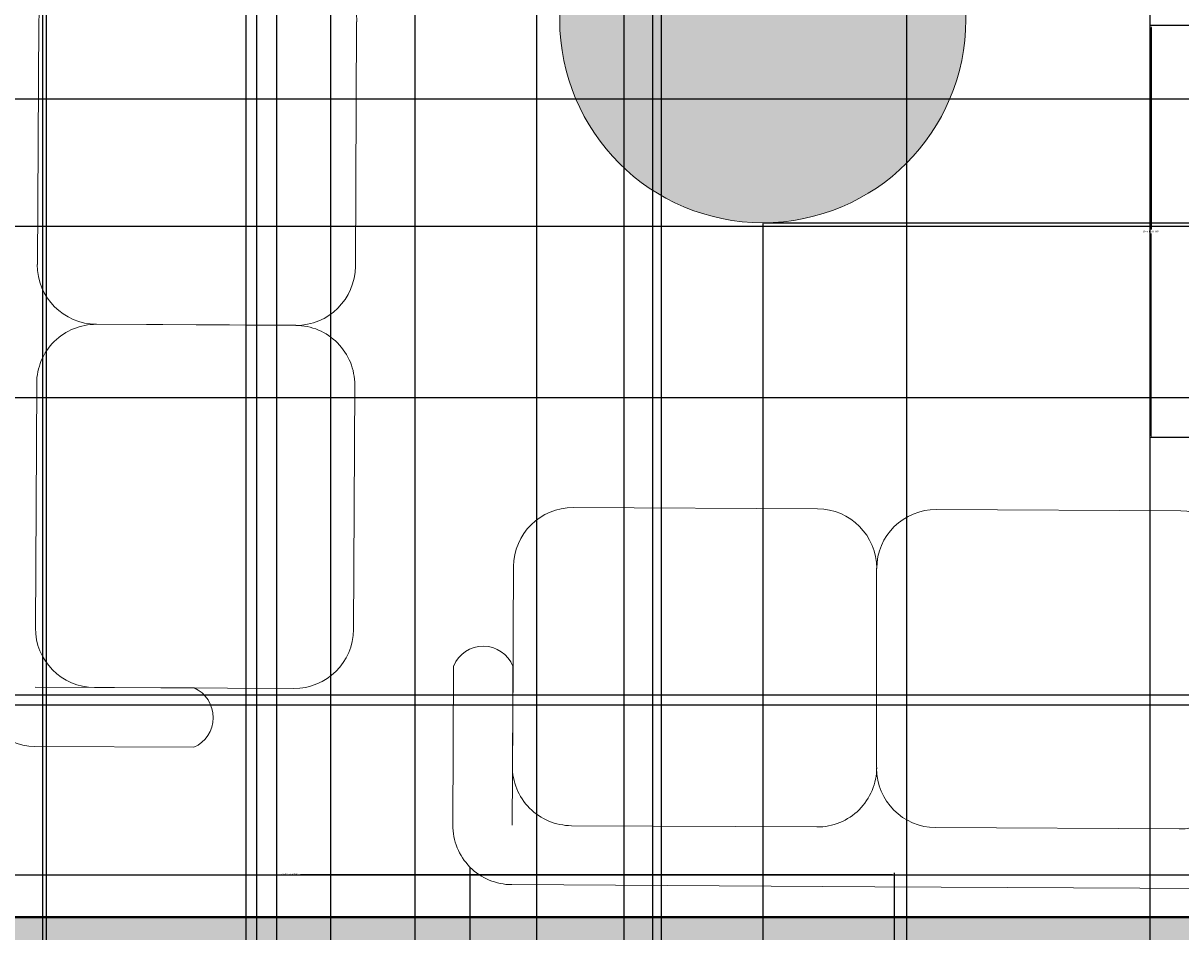
# Model space of a CAD drawing. Units: inches. Extents: x 818 to 1898, y 976 to 2364.
# Tile 32 of 96: x 1282 to 1391, y 1695 to 1780. Entities that reach past the tile are written whole.
import ezdxf

# ---------------------------------------------------------------- set-up
doc = ezdxf.new("R2010")
doc.units = ezdxf.units.IN
doc.header["$LTSCALE"] = 5
doc.header["$MEASUREMENT"] = 0
for name, color, linetype, lineweight in [('A-ANNO-DIMS', 2, 'Continuous', 18), ('A-FLOR-CASE-PATT', 33, 'Continuous', 9), ('A-FURN', 8, 'Continuous', 18), ('A-WALL', 7, 'Continuous', 40)]:
    doc.layers.add(name, color=color, linetype=linetype, lineweight=lineweight)
doc.layers.add('A-WALL-PATT', color=251, linetype='Continuous', lineweight=13, true_color=0x636466)
doc.styles.get("Standard").update_dxf_attribs({"font": 'arial.ttf'})
doc.dimstyles.get("Standard").update_dxf_attribs({"dimtxt": 0.18, "dimasz": 0.18, "dimexe": 0.18, "dimexo": 0.0625, "dimgap": 0.09, "dimtad": 0, "dimtih": 1, "dimtoh": 1, "dimdec": 4, "dimzin": 0, "dimdsep": 46, "dimtxsty": 'Standard', "dimcen": 0.09, "dimadec": 0, "dimazin": 0, "dimtfac": 1, "dimtdec": 4, "dimtofl": 0, "dimtmove": 0, "dimatfit": 3, "dimfxl": 1, "dimtolj": 1, "dimtzin": 0, "dimarcsym": 0})

# ---------------------------------------------------------------- blocks, each defined once
blk = doc.blocks.new('SOFA-3-SEAT')
for p, q in [((39.87, 35.86), (5.7, 36.05)), ((74.05, 35.68), (39.88, 35.86)), ((108.23, 35.49), (74.06, 35.68)), ((0, 15.52), (0.08, 30.49)), ((5.59, 15.49), (5.67, 30.46)), ((34.25, 30.31), (11.25, 30.43)), ((68.34, 30.12), (45.43, 30.24)), ((102.62, 29.94), (79.51, 30.06)), ((108.12, 14.94), (108.2, 29.9)), ((113.71, 14.91), (113.79, 29.87)), ((5.64, 24.87), (5.54, 6.11)), ((39.71, 5.93), (39.81, 24.69)), ((39.82, 24.69), (39.72, 5.93)), ((73.9, 5.71), (73.9, 24.47)), ((108.07, 5.56), (108.17, 24.32)), ((11.09, 0.49), (34.09, 0.37)), ((45.27, 0.31), (68.27, 0.19)), ((79.45, 0.12), (102.45, 0))]:
    blk.add_line(p, q)
for centre, radius, start, end in [((5.67, 30.46), 5.59, 89.6898, 179.6898), ((108.2, 29.9), 5.59, 359.6898, 89.6898), ((11.22, 24.84), 5.59, 89.6898, 179.6898), ((34.22, 24.72), 5.59, 359.6898, 89.6898), ((45.4, 24.66), 5.59, 89.6898, 179.6898), ((68.31, 24.53), 5.59, 0, 89.6898), ((79.48, 24.47), 5.59, 89.6898, 180), ((102.59, 24.35), 5.59, 359.6898, 89.6898), ((2.8, 16.75), 3.06, 203.7099, 335.6698), ((110.92, 16.05), 3.01, 201.7034, 337.6762), ((11.12, 6.08), 5.59, 179.6898, 269.6898), ((34.12, 5.96), 5.59, 269.6898, 359.6898), ((45.3, 5.9), 5.59, 179.6898, 269.6898), ((68.3, 5.77), 5.59, 269.6898, 359.6898), ((79.48, 5.71), 5.59, 179.6898, 269.6898), ((102.48, 5.59), 5.59, 269.6898, 359.6898)]:
    blk.add_arc(centre, radius, start, end)
blk = doc.blocks.new('*D42')
at = {"layer": 'A-ANNO-DIMS', "color": 0, "lineweight": -2, "ltscale": 5, "transparency": 16777216}
for p, q in [((1250.19, 1683.07), (1250.19, 1700.26)), ((1250.37, 1700.08), (1306.12, 1700.08)), ((1363.82, 1700.08), (1308.07, 1700.08)), ((1364, 1683.07), (1364, 1700.26))]:
    blk.add_line(p, q, dxfattribs=at)
at = {"layer": 'A-ANNO-DIMS', "color": 0, "ltscale": 5, "transparency": 16777216}
for points in [[(1250.37, 1700.11), (1250.37, 1700.05), (1250.19, 1700.08)], [(1363.82, 1700.11), (1363.82, 1700.05), (1364, 1700.08)]]:
    blk.add_solid(points, dxfattribs=at)
at = {"layer": 'Defpoints', "color": 0, "ltscale": 5, "transparency": 16777216}
for p in [(1364, 1700.08), (1250.19, 1683.01), (1364, 1683.01)]:
    blk.add_point(p, dxfattribs=at)
at = {"layer": 'A-ANNO-DIMS', "color": 0, "ltscale": 5, "transparency": 16777216, "insert": (1307.1, 1700.08), "char_height": 0.18, "attachment_point": 5}
blk.add_mtext('\\A1;SOFA 114 TYP.', dxfattribs=at)
blk = doc.blocks.new('*D50')
at = {"layer": 'A-ANNO-DIMS', "color": 0, "lineweight": -2, "ltscale": 5, "transparency": 16777216}
for p, q in [((1393.92, 1780.01), (1387.99, 1780.01)), ((1388.17, 1779.83), (1388.17, 1760.8)), ((1388.17, 1741.4), (1388.17, 1760.43)), ((1393.92, 1741.22), (1387.99, 1741.22))]:
    blk.add_line(p, q, dxfattribs=at)
at = {"layer": 'A-ANNO-DIMS', "color": 0, "ltscale": 5, "transparency": 16777216}
for points in [[(1388.14, 1779.83), (1388.2, 1779.83), (1388.17, 1780.01)], [(1388.14, 1741.4), (1388.2, 1741.4), (1388.17, 1741.22)]]:
    blk.add_solid(points, dxfattribs=at)
at = {"layer": 'Defpoints', "color": 0, "ltscale": 5, "transparency": 16777216}
for p in [(1388.17, 1780.01), (1393.99, 1780.01), (1393.99, 1741.22)]:
    blk.add_point(p, dxfattribs=at)
at = {"layer": 'A-ANNO-DIMS', "color": 0, "ltscale": 5, "transparency": 16777216, "insert": (1388.17, 1760.62), "char_height": 0.18, "attachment_point": 5}
blk.add_mtext('\\A1;CHAIR 39 TYP.', dxfattribs=at)
blk = doc.blocks.new('*D61')
at = {"layer": 'A-ANNO-DIMS', "color": 0, "lineweight": -2, "ltscale": 5, "transparency": 16777216}
for p, q in [((1071.73, 1203.03), (1071.73, 2363.87)), ((1071.91, 2363.69), (1250.94, 2363.69)), ((1430.55, 2363.69), (1251.51, 2363.69)), ((1430.73, 1203.03), (1430.73, 2363.87))]:
    blk.add_line(p, q, dxfattribs=at)
at = {"layer": 'A-ANNO-DIMS', "color": 0, "ltscale": 5, "transparency": 16777216}
for points in [[(1071.91, 2363.72), (1071.91, 2363.66), (1071.73, 2363.69)], [(1430.55, 2363.72), (1430.55, 2363.66), (1430.73, 2363.69)]]:
    blk.add_solid(points, dxfattribs=at)
at = {"layer": 'Defpoints', "color": 0, "ltscale": 5, "transparency": 16777216}
for p in [(1430.73, 2363.69), (1071.73, 1202.96), (1430.73, 1202.96)]:
    blk.add_point(p, dxfattribs=at)
at = {"layer": 'A-ANNO-DIMS', "color": 0, "ltscale": 5, "transparency": 16777216, "insert": (1251.23, 2363.69), "char_height": 0.18, "attachment_point": 5}
blk.add_mtext('\\A1;359', dxfattribs=at)
blk = doc.blocks.new('*D64')
at = {"layer": 'A-ANNO-DIMS', "color": 0, "lineweight": -2, "ltscale": 5, "transparency": 16777216}
for p, q in [((1197.73, 1501.14), (1197.73, 2363.87)), ((1197.91, 2363.69), (1313.93, 2363.69)), ((1430.55, 2363.69), (1314.52, 2363.69)), ((1430.73, 1501.14), (1430.73, 2363.87))]:
    blk.add_line(p, q, dxfattribs=at)
at = {"layer": 'A-ANNO-DIMS', "color": 0, "ltscale": 5, "transparency": 16777216}
for points in [[(1197.91, 2363.72), (1197.91, 2363.66), (1197.73, 2363.69)], [(1430.55, 2363.72), (1430.55, 2363.66), (1430.73, 2363.69)]]:
    blk.add_solid(points, dxfattribs=at)
at = {"layer": 'Defpoints', "color": 0, "ltscale": 5, "transparency": 16777216}
for p in [(1430.73, 2363.69), (1197.73, 1501.08), (1430.73, 1501.08)]:
    blk.add_point(p, dxfattribs=at)
at = {"layer": 'A-ANNO-DIMS', "color": 0, "ltscale": 5, "transparency": 16777216, "insert": (1314.23, 2363.69), "char_height": 0.18, "attachment_point": 5}
blk.add_mtext('\\A1;233', dxfattribs=at)
blk = doc.blocks.new('*D85')
at = {"layer": 'A-ANNO-DIMS', "color": 0, "lineweight": -2, "ltscale": 5, "transparency": 16777216}
for p, q in [((1258.79, 2053.08), (1897.92, 2053.08)), ((1897.74, 2052.9), (1897.74, 1876.76)), ((1897.74, 1700.26), (1897.74, 1876.4)), ((1258.79, 1700.08), (1897.92, 1700.08))]:
    blk.add_line(p, q, dxfattribs=at)
at = {"layer": 'A-ANNO-DIMS', "color": 0, "ltscale": 5, "transparency": 16777216}
for points in [[(1897.71, 2052.9), (1897.77, 2052.9), (1897.74, 2053.08)], [(1897.71, 1700.26), (1897.77, 1700.26), (1897.74, 1700.08)]]:
    blk.add_solid(points, dxfattribs=at)
at = {"layer": 'Defpoints', "color": 0, "ltscale": 5, "transparency": 16777216}
for p in [(1258.73, 2053.08), (1897.74, 2053.08), (1258.73, 1700.08)]:
    blk.add_point(p, dxfattribs=at)
at = {"layer": 'A-ANNO-DIMS', "color": 0, "ltscale": 5, "transparency": 16777216, "insert": (1897.74, 1876.58), "char_height": 0.18, "attachment_point": 5}
blk.add_mtext('\\A1;353', dxfattribs=at)
blk = doc.blocks.new('*D96')
at = {"layer": 'A-ANNO-DIMS', "color": 0, "lineweight": -2, "ltscale": 5, "transparency": 16777216}
for p, q in [((1229.65, 1071.12), (1229.65, 2363.87)), ((1229.83, 2363.69), (1256.52, 2363.69)), ((1283.99, 2363.69), (1257.3, 2363.69)), ((1284.17, 1071.12), (1284.17, 2363.87))]:
    blk.add_line(p, q, dxfattribs=at)
at = {"layer": 'A-ANNO-DIMS', "color": 0, "ltscale": 5, "transparency": 16777216}
for points in [[(1229.83, 2363.72), (1229.83, 2363.66), (1229.65, 2363.69)], [(1283.99, 2363.72), (1283.99, 2363.66), (1284.17, 2363.69)]]:
    blk.add_solid(points, dxfattribs=at)
at = {"layer": 'Defpoints', "color": 0, "ltscale": 5, "transparency": 16777216}
for p in [(1284.17, 2363.69), (1229.65, 1071.06), (1284.17, 1071.06)]:
    blk.add_point(p, dxfattribs=at)
at = {"layer": 'A-ANNO-DIMS', "color": 0, "ltscale": 5, "transparency": 16777216, "insert": (1256.91, 2363.69), "char_height": 0.18, "attachment_point": 5}
blk.add_mtext('\\A1;54.52', dxfattribs=at)
blk = doc.blocks.new('*D97')
at = {"layer": 'A-ANNO-DIMS', "color": 0, "lineweight": -2, "ltscale": 5, "transparency": 16777216}
for p, q in [((1284.17, 1071.12), (1284.17, 2363.87)), ((1284.35, 2363.69), (1310.96, 2363.69)), ((1338.36, 2363.69), (1311.75, 2363.69)), ((1338.54, 1071.12), (1338.54, 2363.87))]:
    blk.add_line(p, q, dxfattribs=at)
at = {"layer": 'A-ANNO-DIMS', "color": 0, "ltscale": 5, "transparency": 16777216}
for points in [[(1284.35, 2363.72), (1284.35, 2363.66), (1284.17, 2363.69)], [(1338.36, 2363.72), (1338.36, 2363.66), (1338.54, 2363.69)]]:
    blk.add_solid(points, dxfattribs=at)
at = {"layer": 'Defpoints', "color": 0, "ltscale": 5, "transparency": 16777216}
for p in [(1338.54, 2363.69), (1284.17, 1071.06), (1338.54, 1071.06)]:
    blk.add_point(p, dxfattribs=at)
at = {"layer": 'A-ANNO-DIMS', "color": 0, "ltscale": 5, "transparency": 16777216, "insert": (1311.36, 2363.69), "char_height": 0.18, "attachment_point": 5}
blk.add_mtext('\\A1;54.37', dxfattribs=at)
blk = doc.blocks.new('*D98')
at = {"layer": 'A-ANNO-DIMS', "color": 0, "lineweight": -2, "ltscale": 5, "transparency": 16777216}
for p, q in [((1338.54, 1071.12), (1338.54, 2363.87)), ((1338.72, 2363.69), (1364.81, 2363.69)), ((1391.7, 2363.69), (1365.6, 2363.69)), ((1391.88, 1071.12), (1391.88, 2363.87))]:
    blk.add_line(p, q, dxfattribs=at)
at = {"layer": 'A-ANNO-DIMS', "color": 0, "ltscale": 5, "transparency": 16777216}
for points in [[(1338.72, 2363.72), (1338.72, 2363.66), (1338.54, 2363.69)], [(1391.7, 2363.72), (1391.7, 2363.66), (1391.88, 2363.69)]]:
    blk.add_solid(points, dxfattribs=at)
at = {"layer": 'Defpoints', "color": 0, "ltscale": 5, "transparency": 16777216}
for p in [(1391.88, 2363.69), (1338.54, 1071.06), (1391.88, 1071.06)]:
    blk.add_point(p, dxfattribs=at)
at = {"layer": 'A-ANNO-DIMS', "color": 0, "ltscale": 5, "transparency": 16777216, "insert": (1365.21, 2363.69), "char_height": 0.18, "attachment_point": 5}
blk.add_mtext('\\A1;53.33', dxfattribs=at)
blk = doc.blocks.new('*D119')
at = {"layer": 'A-ANNO-DIMS', "color": 0, "lineweight": -2, "ltscale": 5, "transparency": 16777216}
for p, q in [((1766.29, 1716.99), (818.03, 1716.99)), ((818.21, 1716.81), (818.21, 1672.43)), ((818.21, 1627.69), (818.21, 1672.06)), ((1766.29, 1627.51), (818.03, 1627.51))]:
    blk.add_line(p, q, dxfattribs=at)
at = {"layer": 'A-ANNO-DIMS', "color": 0, "ltscale": 5, "transparency": 16777216}
for points in [[(818.18, 1716.81), (818.24, 1716.81), (818.21, 1716.99)], [(818.18, 1627.69), (818.24, 1627.69), (818.21, 1627.51)]]:
    blk.add_solid(points, dxfattribs=at)
at = {"layer": 'Defpoints', "color": 0, "ltscale": 5, "transparency": 16777216}
for p in [(818.21, 1716.99), (1766.35, 1716.99), (1766.35, 1627.51)]:
    blk.add_point(p, dxfattribs=at)
at = {"layer": 'A-ANNO-DIMS', "color": 0, "ltscale": 5, "transparency": 16777216, "insert": (818.21, 1672.25), "char_height": 0.18, "attachment_point": 5}
blk.add_mtext('\\A1;89.48', dxfattribs=at)
blk = doc.blocks.new('*D120')
at = {"layer": 'A-ANNO-DIMS', "color": 0, "lineweight": -2, "ltscale": 5, "transparency": 16777216}
for p, q in [((1766.29, 1797.72), (818.03, 1797.72)), ((818.21, 1797.54), (818.21, 1757.53)), ((818.21, 1717.17), (818.21, 1757.17)), ((1766.29, 1716.99), (818.03, 1716.99))]:
    blk.add_line(p, q, dxfattribs=at)
at = {"layer": 'A-ANNO-DIMS', "color": 0, "ltscale": 5, "transparency": 16777216}
for points in [[(818.18, 1797.54), (818.24, 1797.54), (818.21, 1797.72)], [(818.18, 1717.17), (818.24, 1717.17), (818.21, 1716.99)]]:
    blk.add_solid(points, dxfattribs=at)
at = {"layer": 'Defpoints', "color": 0, "ltscale": 5, "transparency": 16777216}
for p in [(818.21, 1797.72), (1766.35, 1797.72), (1766.35, 1716.99)]:
    blk.add_point(p, dxfattribs=at)
at = {"layer": 'A-ANNO-DIMS', "color": 0, "ltscale": 5, "transparency": 16777216, "insert": (818.21, 1757.35), "char_height": 0.18, "attachment_point": 5}
blk.add_mtext('\\A1;80.73', dxfattribs=at)
blk = doc.blocks.new('*D165')
at = {"layer": 'A-ANNO-DIMS', "color": 0, "lineweight": -2, "ltscale": 5, "transparency": 16777216}
for p, q in [((1283.82, 1510.14), (1283.82, 2363.87)), ((1284, 2363.69), (1324.09, 2363.69)), ((1364.97, 2363.69), (1324.88, 2363.69)), ((1365.15, 1510.14), (1365.15, 2363.87))]:
    blk.add_line(p, q, dxfattribs=at)
at = {"layer": 'A-ANNO-DIMS', "color": 0, "ltscale": 5, "transparency": 16777216}
for points in [[(1284, 2363.72), (1284, 2363.66), (1283.82, 2363.69)], [(1364.97, 2363.72), (1364.97, 2363.66), (1365.15, 2363.69)]]:
    blk.add_solid(points, dxfattribs=at)
at = {"layer": 'Defpoints', "color": 0, "ltscale": 5, "transparency": 16777216}
for p in [(1365.15, 2363.69), (1283.82, 1510.08), (1365.15, 1510.08)]:
    blk.add_point(p, dxfattribs=at)
at = {"layer": 'A-ANNO-DIMS', "color": 0, "ltscale": 5, "transparency": 16777216, "insert": (1324.48, 2363.69), "char_height": 0.18, "attachment_point": 5}
blk.add_mtext('\\A1;81.33', dxfattribs=at)
blk = doc.blocks.new('*D215')
at = {"layer": 'A-ANNO-DIMS', "color": 0, "lineweight": -2, "ltscale": 5, "transparency": 16777216}
for p, q in [((1590.66, 1876.08), (818.03, 1876.08)), ((818.21, 1875.9), (818.21, 1781.76)), ((818.21, 1687.26), (818.21, 1781.4)), ((1511.66, 1687.08), (818.03, 1687.08))]:
    blk.add_line(p, q, dxfattribs=at)
at = {"layer": 'A-ANNO-DIMS', "color": 0, "ltscale": 5, "transparency": 16777216}
for points in [[(818.18, 1875.9), (818.24, 1875.9), (818.21, 1876.08)], [(818.18, 1687.26), (818.24, 1687.26), (818.21, 1687.08)]]:
    blk.add_solid(points, dxfattribs=at)
at = {"layer": 'Defpoints', "color": 0, "ltscale": 5, "transparency": 16777216}
for p in [(818.21, 1876.08), (1590.73, 1876.08), (1511.73, 1687.08)]:
    blk.add_point(p, dxfattribs=at)
at = {"layer": 'A-ANNO-DIMS', "color": 0, "ltscale": 5, "transparency": 16777216, "insert": (818.21, 1781.58), "char_height": 0.18, "attachment_point": 5}
blk.add_mtext('\\A1;189', dxfattribs=at)
blk = doc.blocks.new('*D220')
at = {"layer": 'A-ANNO-DIMS', "color": 0, "lineweight": -2, "ltscale": 5, "transparency": 16777216}
for p, q in [((1520.66, 1773.08), (818.03, 1773.08)), ((818.21, 1772.9), (818.21, 1767.26)), ((818.21, 1761.26), (818.21, 1766.9)), ((1520.66, 1761.08), (818.03, 1761.08))]:
    blk.add_line(p, q, dxfattribs=at)
at = {"layer": 'A-ANNO-DIMS', "color": 0, "ltscale": 5, "transparency": 16777216}
for points in [[(818.18, 1772.9), (818.24, 1772.9), (818.21, 1773.08)], [(818.18, 1761.26), (818.24, 1761.26), (818.21, 1761.08)]]:
    blk.add_solid(points, dxfattribs=at)
at = {"layer": 'Defpoints', "color": 0, "ltscale": 5, "transparency": 16777216}
for p in [(818.21, 1773.08), (1520.73, 1773.08), (1520.73, 1761.08)]:
    blk.add_point(p, dxfattribs=at)
at = {"layer": 'A-ANNO-DIMS', "color": 0, "ltscale": 5, "transparency": 16777216, "insert": (818.21, 1767.08), "char_height": 0.18, "attachment_point": 5}
blk.add_mtext('\\A1;12', dxfattribs=at)
blk = doc.blocks.new('*D222')
at = {"layer": 'A-ANNO-DIMS', "color": 0, "lineweight": -2, "ltscale": 5, "transparency": 16777216}
for p, q in [((1511.66, 1744.97), (818.03, 1744.97)), ((818.21, 1744.79), (818.21, 1730.69)), ((818.21, 1716.23), (818.21, 1730.33)), ((1511.66, 1716.05), (818.03, 1716.05))]:
    blk.add_line(p, q, dxfattribs=at)
at = {"layer": 'A-ANNO-DIMS', "color": 0, "ltscale": 5, "transparency": 16777216}
for points in [[(818.18, 1744.79), (818.24, 1744.79), (818.21, 1744.97)], [(818.18, 1716.23), (818.24, 1716.23), (818.21, 1716.05)]]:
    blk.add_solid(points, dxfattribs=at)
at = {"layer": 'Defpoints', "color": 0, "ltscale": 5, "transparency": 16777216}
for p in [(818.21, 1744.97), (1511.73, 1744.97), (1511.73, 1716.05)]:
    blk.add_point(p, dxfattribs=at)
at = {"layer": 'A-ANNO-DIMS', "color": 0, "ltscale": 5, "transparency": 16777216, "insert": (818.21, 1730.51), "char_height": 0.18, "attachment_point": 5}
blk.add_mtext('\\A1;28.926', dxfattribs=at)
blk = doc.blocks.new('*D223')
at = {"layer": 'A-ANNO-DIMS', "color": 0, "lineweight": -2, "ltscale": 5, "transparency": 16777216}
for p, q in [((1511.66, 1716.05), (818.03, 1716.05)), ((818.21, 1715.87), (818.21, 1706.24)), ((818.21, 1696.26), (818.21, 1705.88)), ((1511.66, 1696.08), (818.03, 1696.08))]:
    blk.add_line(p, q, dxfattribs=at)
at = {"layer": 'A-ANNO-DIMS', "color": 0, "ltscale": 5, "transparency": 16777216}
for points in [[(818.18, 1715.87), (818.24, 1715.87), (818.21, 1716.05)], [(818.18, 1696.26), (818.24, 1696.26), (818.21, 1696.08)]]:
    blk.add_solid(points, dxfattribs=at)
at = {"layer": 'Defpoints', "color": 0, "ltscale": 5, "transparency": 16777216}
for p in [(818.21, 1716.05), (1511.73, 1716.05), (1511.73, 1696.08)]:
    blk.add_point(p, dxfattribs=at)
at = {"layer": 'A-ANNO-DIMS', "color": 0, "ltscale": 5, "transparency": 16777216, "insert": (818.21, 1706.06), "char_height": 0.18, "attachment_point": 5}
blk.add_mtext('\\A1;19.967', dxfattribs=at)
blk = doc.blocks.new('*D231')
at = {"layer": 'A-ANNO-DIMS', "color": 0, "lineweight": -2, "ltscale": 5, "transparency": 16777216}
for p, q in [((1303.93, 1952.98), (1303.93, 975.66)), ((1402.52, 1952.98), (1402.52, 975.66)), ((1304.11, 975.84), (1352.83, 975.84)), ((1402.34, 975.84), (1353.62, 975.84))]:
    blk.add_line(p, q, dxfattribs=at)
at = {"layer": 'A-ANNO-DIMS', "color": 0, "ltscale": 5, "transparency": 16777216}
for points in [[(1304.11, 975.87), (1304.11, 975.81), (1303.93, 975.84)], [(1402.34, 975.87), (1402.34, 975.81), (1402.52, 975.84)]]:
    blk.add_solid(points, dxfattribs=at)
at = {"layer": 'Defpoints', "color": 0, "ltscale": 5, "transparency": 16777216}
for p in [(1303.93, 1953.04), (1402.52, 1953.04), (1402.52, 975.84)]:
    blk.add_point(p, dxfattribs=at)
at = {"layer": 'A-ANNO-DIMS', "color": 0, "ltscale": 5, "transparency": 16777216, "insert": (1353.22, 975.84), "char_height": 0.18, "attachment_point": 5}
blk.add_mtext('\\A1;98.59', dxfattribs=at)
blk = doc.blocks.new('*D233')
at = {"layer": 'A-ANNO-DIMS', "color": 0, "lineweight": -2, "ltscale": 5, "transparency": 16777216}
for p, q in [((1267.73, 2044.02), (1267.73, 975.66)), ((1303.93, 2008.33), (1303.93, 975.66)), ((1267.91, 975.84), (1285.36, 975.84)), ((1303.75, 975.84), (1286.29, 975.84))]:
    blk.add_line(p, q, dxfattribs=at)
at = {"layer": 'A-ANNO-DIMS', "color": 0, "ltscale": 5, "transparency": 16777216}
for points in [[(1267.91, 975.87), (1267.91, 975.81), (1267.73, 975.84)], [(1303.75, 975.87), (1303.75, 975.81), (1303.93, 975.84)]]:
    blk.add_solid(points, dxfattribs=at)
at = {"layer": 'Defpoints', "color": 0, "ltscale": 5, "transparency": 16777216}
for p in [(1267.73, 2044.08), (1303.93, 2008.39), (1303.93, 975.84)]:
    blk.add_point(p, dxfattribs=at)
at = {"layer": 'A-ANNO-DIMS', "color": 0, "ltscale": 5, "transparency": 16777216, "insert": (1285.83, 975.84), "char_height": 0.18, "attachment_point": 5}
blk.add_mtext('\\A1;36.206', dxfattribs=at)
blk = doc.blocks.new('*D236')
at = {"layer": 'A-ANNO-DIMS', "color": 0, "lineweight": -2, "ltscale": 5, "transparency": 16777216}
for p, q in [((1310.91, 2026.14), (1310.91, 975.66)), ((1342.04, 2026.14), (1342.04, 975.66)), ((1311.09, 975.84), (1326.08, 975.84)), ((1341.86, 975.84), (1326.87, 975.84))]:
    blk.add_line(p, q, dxfattribs=at)
at = {"layer": 'A-ANNO-DIMS', "color": 0, "ltscale": 5, "transparency": 16777216}
for points in [[(1311.09, 975.87), (1311.09, 975.81), (1310.91, 975.84)], [(1341.86, 975.87), (1341.86, 975.81), (1342.04, 975.84)]]:
    blk.add_solid(points, dxfattribs=at)
at = {"layer": 'Defpoints', "color": 0, "ltscale": 5, "transparency": 16777216}
for p in [(1310.91, 2026.21), (1342.04, 2026.21), (1342.04, 975.84)]:
    blk.add_point(p, dxfattribs=at)
at = {"layer": 'A-ANNO-DIMS', "color": 0, "ltscale": 5, "transparency": 16777216, "insert": (1326.48, 975.84), "char_height": 0.18, "attachment_point": 5}
blk.add_mtext('\\A1;31.14', dxfattribs=at)
blk = doc.blocks.new('*D252')
at = {"layer": 'A-ANNO-DIMS', "color": 0, "lineweight": -2, "ltscale": 5, "transparency": 16777216}
for p, q in [((1330.3, 2053.02), (1330.3, 975.66)), ((1388.03, 2053.02), (1388.03, 975.66)), ((1330.48, 975.84), (1358.77, 975.84)), ((1387.85, 975.84), (1359.56, 975.84))]:
    blk.add_line(p, q, dxfattribs=at)
at = {"layer": 'A-ANNO-DIMS', "color": 0, "ltscale": 5, "transparency": 16777216}
for points in [[(1330.48, 975.87), (1330.48, 975.81), (1330.3, 975.84)], [(1387.85, 975.87), (1387.85, 975.81), (1388.03, 975.84)]]:
    blk.add_solid(points, dxfattribs=at)
at = {"layer": 'Defpoints', "color": 0, "ltscale": 5, "transparency": 16777216}
for p in [(1330.3, 2053.08), (1388.03, 2053.08), (1388.03, 975.84)]:
    blk.add_point(p, dxfattribs=at)
at = {"layer": 'A-ANNO-DIMS', "color": 0, "ltscale": 5, "transparency": 16777216, "insert": (1359.17, 975.84), "char_height": 0.18, "attachment_point": 5}
blk.add_mtext('\\A1;57.73', dxfattribs=at)
blk = doc.blocks.new('*D254')
at = {"layer": 'A-ANNO-DIMS', "color": 0, "lineweight": -2, "ltscale": 5, "transparency": 16777216}
for p, q in [((1267.73, 2044.02), (1267.73, 975.66)), ((1330.3, 2044.02), (1330.3, 975.66)), ((1267.91, 975.84), (1298.62, 975.84)), ((1330.12, 975.84), (1299.41, 975.84))]:
    blk.add_line(p, q, dxfattribs=at)
at = {"layer": 'A-ANNO-DIMS', "color": 0, "ltscale": 5, "transparency": 16777216}
for points in [[(1267.91, 975.87), (1267.91, 975.81), (1267.73, 975.84)], [(1330.12, 975.87), (1330.12, 975.81), (1330.3, 975.84)]]:
    blk.add_solid(points, dxfattribs=at)
at = {"layer": 'Defpoints', "color": 0, "ltscale": 5, "transparency": 16777216}
for p in [(1267.73, 2044.08), (1330.3, 2044.08), (1330.3, 975.84)]:
    blk.add_point(p, dxfattribs=at)
at = {"layer": 'A-ANNO-DIMS', "color": 0, "ltscale": 5, "transparency": 16777216, "insert": (1299.02, 975.84), "char_height": 0.18, "attachment_point": 5}
blk.add_mtext('\\A1;62.58', dxfattribs=at)
blk = doc.blocks.new('*D269')
at = {"layer": 'A-ANNO-DIMS', "color": 0, "lineweight": -2, "ltscale": 5, "transparency": 16777216}
for p, q in [((1246.94, 1534.14), (1246.94, 2363.87)), ((1247.12, 2363.69), (1293.71, 2363.69)), ((1341.08, 2363.69), (1294.49, 2363.69)), ((1341.26, 1534.14), (1341.26, 2363.87))]:
    blk.add_line(p, q, dxfattribs=at)
at = {"layer": 'A-ANNO-DIMS', "color": 0, "ltscale": 5, "transparency": 16777216}
for points in [[(1247.12, 2363.72), (1247.12, 2363.66), (1246.94, 2363.69)], [(1341.08, 2363.72), (1341.08, 2363.66), (1341.26, 2363.69)]]:
    blk.add_solid(points, dxfattribs=at)
at = {"layer": 'Defpoints', "color": 0, "ltscale": 5, "transparency": 16777216}
for p in [(1341.26, 2363.69), (1246.94, 1534.08), (1341.26, 1534.08)]:
    blk.add_point(p, dxfattribs=at)
at = {"layer": 'A-ANNO-DIMS', "color": 0, "ltscale": 5, "transparency": 16777216, "insert": (1294.1, 2363.69), "char_height": 0.18, "attachment_point": 5}
blk.add_mtext('\\A1;94.32', dxfattribs=at)
blk = doc.blocks.new('*D278')
at = {"layer": 'A-ANNO-DIMS', "color": 0, "lineweight": -2, "ltscale": 5, "transparency": 16777216}
for p, q in [((1324.03, 1700.74), (1324.03, 975.66)), ((1267.73, 1696.02), (1267.73, 975.66)), ((1267.91, 975.84), (1295.5, 975.84)), ((1323.85, 975.84), (1296.26, 975.84))]:
    blk.add_line(p, q, dxfattribs=at)
at = {"layer": 'A-ANNO-DIMS', "color": 0, "ltscale": 5, "transparency": 16777216}
for points in [[(1267.91, 975.87), (1267.91, 975.81), (1267.73, 975.84)], [(1323.85, 975.87), (1323.85, 975.81), (1324.03, 975.84)]]:
    blk.add_solid(points, dxfattribs=at)
at = {"layer": 'Defpoints', "color": 0, "ltscale": 5, "transparency": 16777216}
for p in [(1324.03, 1700.81), (1267.73, 1696.08), (1324.03, 975.84)]:
    blk.add_point(p, dxfattribs=at)
at = {"layer": 'A-ANNO-DIMS', "color": 0, "ltscale": 5, "transparency": 16777216, "insert": (1295.88, 975.84), "char_height": 0.18, "attachment_point": 5}
blk.add_mtext('\\A1;56.31', dxfattribs=at)
blk = doc.blocks.new('*D283')
at = {"layer": 'A-ANNO-DIMS', "color": 0, "lineweight": -2, "ltscale": 5, "transparency": 16777216}
for p, q in [((1351.6, 1761.39), (1351.6, 975.66)), ((1267.73, 1696.02), (1267.73, 975.66)), ((1267.91, 975.84), (1309.27, 975.84)), ((1351.42, 975.84), (1310.06, 975.84))]:
    blk.add_line(p, q, dxfattribs=at)
at = {"layer": 'A-ANNO-DIMS', "color": 0, "ltscale": 5, "transparency": 16777216}
for points in [[(1267.91, 975.87), (1267.91, 975.81), (1267.73, 975.84)], [(1351.42, 975.87), (1351.42, 975.81), (1351.6, 975.84)]]:
    blk.add_solid(points, dxfattribs=at)
at = {"layer": 'Defpoints', "color": 0, "ltscale": 5, "transparency": 16777216}
for p in [(1351.6, 1761.45), (1267.73, 1696.08), (1351.6, 975.84)]:
    blk.add_point(p, dxfattribs=at)
at = {"layer": 'A-ANNO-DIMS', "color": 0, "ltscale": 5, "transparency": 16777216, "insert": (1309.66, 975.84), "char_height": 0.18, "attachment_point": 5}
blk.add_mtext('\\A1;83.87', dxfattribs=at)
blk = doc.blocks.new('*D284')
at = {"layer": 'A-ANNO-DIMS', "color": 0, "lineweight": -2, "ltscale": 5, "transparency": 16777216}
for p, q in [((1351.66, 1761.45), (1897.92, 1761.45)), ((1897.74, 1761.27), (1897.74, 1728.95)), ((1897.74, 1696.26), (1897.74, 1728.58)), ((1267.79, 1696.08), (1897.92, 1696.08))]:
    blk.add_line(p, q, dxfattribs=at)
at = {"layer": 'A-ANNO-DIMS', "color": 0, "ltscale": 5, "transparency": 16777216}
for points in [[(1897.71, 1761.27), (1897.77, 1761.27), (1897.74, 1761.45)], [(1897.71, 1696.26), (1897.77, 1696.26), (1897.74, 1696.08)]]:
    blk.add_solid(points, dxfattribs=at)
at = {"layer": 'Defpoints', "color": 0, "ltscale": 5, "transparency": 16777216}
for p in [(1351.6, 1761.45), (1267.73, 1696.08), (1897.74, 1696.08)]:
    blk.add_point(p, dxfattribs=at)
at = {"layer": 'A-ANNO-DIMS', "color": 0, "ltscale": 5, "transparency": 16777216, "insert": (1897.74, 1728.76), "char_height": 0.18, "attachment_point": 5}
blk.add_mtext('\\A1;65.37', dxfattribs=at)
blk = doc.blocks.new('*D285')
at = {"layer": 'A-ANNO-DIMS', "color": 0, "lineweight": -2, "ltscale": 5, "transparency": 16777216}
for p, q in [((1305.83, 1830.02), (1305.83, 975.66)), ((1267.73, 1814.9), (1267.73, 975.66)), ((1267.91, 975.84), (1286.47, 975.84)), ((1305.65, 975.84), (1287.08, 975.84))]:
    blk.add_line(p, q, dxfattribs=at)
at = {"layer": 'A-ANNO-DIMS', "color": 0, "ltscale": 5, "transparency": 16777216}
for points in [[(1267.91, 975.87), (1267.91, 975.81), (1267.73, 975.84)], [(1305.65, 975.87), (1305.65, 975.81), (1305.83, 975.84)]]:
    blk.add_solid(points, dxfattribs=at)
at = {"layer": 'Defpoints', "color": 0, "ltscale": 5, "transparency": 16777216}
for p in [(1305.83, 1830.08), (1267.73, 1814.97), (1267.73, 975.84)]:
    blk.add_point(p, dxfattribs=at)
at = {"layer": 'A-ANNO-DIMS', "color": 0, "ltscale": 5, "transparency": 16777216, "insert": (1286.78, 975.84), "char_height": 0.18, "attachment_point": 5}
blk.add_mtext('\\A1;38.1', dxfattribs=at)
blk = doc.blocks.new('*D290')
at = {"layer": 'A-ANNO-DIMS', "color": 0, "lineweight": -2, "ltscale": 5, "transparency": 16777216}
for p, q in [((1302.98, 1599.43), (1302.98, 2363.87)), ((1303.16, 2363.69), (1310.57, 2363.69)), ((1318.71, 2363.69), (1311.31, 2363.69)), ((1318.89, 1607.83), (1318.89, 2363.87))]:
    blk.add_line(p, q, dxfattribs=at)
at = {"layer": 'A-ANNO-DIMS', "color": 0, "ltscale": 5, "transparency": 16777216}
for points in [[(1303.16, 2363.72), (1303.16, 2363.66), (1302.98, 2363.69)], [(1318.71, 2363.72), (1318.71, 2363.66), (1318.89, 2363.69)]]:
    blk.add_solid(points, dxfattribs=at)
at = {"layer": 'Defpoints', "color": 0, "ltscale": 5, "transparency": 16777216}
for p in [(1318.89, 2363.69), (1318.89, 1607.77), (1302.98, 1599.37)]:
    blk.add_point(p, dxfattribs=at)
at = {"layer": 'A-ANNO-DIMS', "color": 0, "ltscale": 5, "transparency": 16777216, "insert": (1310.94, 2363.69), "char_height": 0.18, "attachment_point": 5}
blk.add_mtext('\\A1;15.91', dxfattribs=at)

msp = doc.modelspace()

# ---------------------------------------------------------------- hatches: boundary and pattern name
at = {"layer": 'A-FLOR-CASE-PATT', "ltscale": 5}
h = msp.add_hatch(color=256, dxfattribs=at)
h.dxf.hatch_style = 1
h.paths.add_polyline_path([(1705.7252, 1941.0782), (1681.7252, 1941.0782), (1681.7252, 1900.0782), (1599.7252, 1900.0782), (1599.7252, 1876.0782), (1705.7252, 1876.0782)])
h.paths.add_polyline_path([(1457.7252, 1409.1177), (1457.7252, 1526.6712), (1439.7252, 1526.6712), (1439.7252, 1457.5313), (1446.3307, 1457.5313), (1446.3307, 1468.9514), (1446.8307, 1470.665), (1446.8307, 1469.665), (1446.8307, 1468.9514), (1446.8307, 1456.8361), (1446.8307, 1444.7258), (1446.8307, 1443.3338), (1446.3307, 1444.7258), (1446.3307, 1456.8361), (1439.7252, 1456.8361), (1439.7252, 1355.0782), (1463.7252, 1355.0782), (1463.7252, 1367.3287), (1458.0475, 1367.3287, -0.23606798), (1457.0475, 1369.3287), (1456.0475, 1369.3287, -0.11764706), (1456.0475, 1386.3287), (1457.0475, 1386.3287, -0.23606798), (1458.0475, 1388.3287), (1463.7252, 1388.3287), (1463.7252, 1389.3211)])
h.paths.add_polyline_path([(1341.2593, 1534.0782), (1246.9377, 1534.0782), (1246.9377, 1510.0782), (1341.2593, 1510.0782)])
h.paths.add_polyline_path([(1288.8272, 1519.927), (1289.8272, 1519.927), (1290.5408, 1519.927), (1302.6561, 1519.927), (1314.7664, 1519.927), (1316.1584, 1519.927), (1314.7664, 1519.427), (1302.6561, 1519.427), (1302.6561, 1512.8214), (1301.9609, 1512.8214), (1301.9609, 1519.427), (1290.5408, 1519.427)], flags=16)
h.paths.add_polyline_path([(1377.7791, 1867.0782), (1344.5531, 1867.0782), (1344.5531, 1860.4726), (1355.9731, 1860.4726), (1357.6867, 1859.9726), (1356.6867, 1859.9726), (1355.9731, 1859.9726), (1343.8579, 1859.9726), (1331.7475, 1859.9726), (1330.3556, 1859.9726), (1331.7475, 1860.4726), (1343.8579, 1860.4726), (1343.8579, 1867.0782), (1311.3271, 1867.0782), (1311.3271, 1853.7496), (1377.7791, 1853.7496)])
h.paths.add_polyline_path([(1301.148, 1610.7299, -0.46196039), (1314.4882, 1599.3725, -0.19222541), (1311.3254, 1591.4497, 0.54791519), (1336.8832, 1607.7707, 0.92061359)])
h.paths.add_polyline_path([(1370.719, 1780.5695, 1), (1332.478, 1780.5695, 1)])
h.paths.add_polyline_path([(1705.7252, 1463.0782), (1681.7252, 1463.0782), (1681.7252, 1379.0782), (1622.7252, 1379.0782), (1622.7252, 1355.0782), (1705.7252, 1355.0782)])
h.paths.add_polyline_path([(1658.1052, 1359.2188), (1658.1786, 1359.2188), (1658.1786, 1373.8763), (1658.1052, 1373.9202)], flags=16)
h.paths.add_polyline_path([(1686.9271, 1409.9311), (1686.8832, 1409.8578), (1701.5845, 1409.8578), (1701.5845, 1409.9311)], flags=16)
h.paths.add_polyline_path([(1637.1266, 1359.2188), (1637.2, 1359.2188), (1637.2, 1373.8763), (1637.1266, 1373.9202)], flags=16)
at = {"layer": 'A-WALL-PATT', "ltscale": 5}
h = msp.add_hatch(color=256, dxfattribs=at)
h.dxf.hatch_style = 1
h.paths.add_polyline_path([(1267.7251, 1928.9218), (1258.7251, 1928.9218), (1258.7251, 1913.6401), (1250.3029, 1913.6401), (1250.3029, 1878.3919), (1258.7251, 1878.3919), (1258.7251, 1862.9652), (1267.7251, 1862.9652)])
h.paths.add_polyline_path([(1267.7251, 1814.9652), (1258.7251, 1814.9652), (1258.7251, 1755.3321), (1267.7251, 1755.3321)])
h.paths.add_polyline_path([(1463.7252, 1696.0782), (1267.7251, 1696.0782), (1267.7251, 1707.3321), (1258.7251, 1707.3321), (1258.7251, 1700.0782), (1251.9333, 1700.0782), (1251.9333, 1687.0782), (1463.7252, 1687.0782)])
h.paths.add_polyline_path([(1714.7252, 1717.3178), (1705.7252, 1717.3178), (1705.7252, 1696.0782), (1599.7252, 1696.0782), (1599.7252, 1790.0782), (1705.7252, 1790.0782), (1705.7252, 1785.6125), (1714.7252, 1785.6125), (1714.7252, 1827.2125), (1705.7252, 1827.2125), (1705.7252, 1802.0782), (1599.7252, 1802.0782), (1599.7252, 1867.0782), (1705.7252, 1867.0782), (1705.7252, 1857.2125), (1714.7252, 1857.2125), (1714.7252, 1930.0316), (1741.8409, 1930.0316), (1741.8409, 1935.0316), (1714.7252, 1935.0316), (1714.7252, 1957.0338), (1741.8409, 1957.0338), (1741.8409, 1962.0338), (1714.7252, 1962.0338), (1705.7252, 1962.0338), (1705.7252, 1948.0782), (1599.7252, 1948.0782), (1599.7252, 1981.0782), (1590.7251, 1981.0782), (1590.7251, 1941.0782), (1620.7252, 1941.0782), (1705.7252, 1941.0782), (1705.7252, 1876.0782), (1599.7252, 1876.0782), (1599.7252, 1911.0782), (1590.7251, 1911.0782), (1590.7251, 1876.0782), (1429.2252, 1876.0782), (1429.2252, 1867.0782), (1511.7251, 1867.0782), (1528.593, 1867.0782), (1595.7252, 1867.0782), (1595.7252, 1773.0782), (1520.7251, 1773.0782), (1520.7251, 1837.5823), (1532.593, 1837.5823), (1532.593, 1867.0782), (1528.593, 1867.0782), (1528.593, 1841.5823), (1511.7251, 1841.5823), (1511.7251, 1744.9714), (1520.7251, 1744.9714), (1520.7251, 1761.0782), (1595.7252, 1761.0782), (1595.7252, 1696.0782), (1520.7251, 1696.0782), (1520.7251, 1716.0454), (1511.7251, 1716.0454), (1511.7251, 1696.0782), (1511.7251, 1687.0782), (1714.7252, 1687.0782)])
h.paths.add_polyline_path([(1714.7252, 2053.0782), (1714.7252, 2081.1881), (1709.7252, 2081.1881), (1709.7252, 2053.0782), (1681.6446, 2053.0782), (1681.6446, 2081.1881), (1676.6446, 2081.1881), (1676.6446, 2053.0782), (1538.5155, 2053.0782), (1538.5155, 2044.0782), (1590.7251, 2044.0782), (1590.7251, 2011.0782), (1599.7252, 2011.0782), (1599.7252, 2044.0782), (1705.7252, 2044.0782), (1705.7252, 2014.5114), (1714.7252, 2014.5114)])
h.paths.add_polyline_path([(1485.1216, 2053.0782), (1422.02, 2053.0782), (1422.02, 2081.1881), (1413.02, 2081.1881), (1413.02, 2053.0782), (1399.6356, 2053.0782), (1399.6356, 2081.1881), (1390.6356, 2081.1881), (1390.6356, 2053.0782), (1388.0315, 2053.0782), (1388.0315, 2044.0782), (1416.2743, 2044.0782), (1485.1216, 2044.0782)])
h.paths.add_polyline_path([(1330.305, 2053.0782), (1258.7251, 2053.0782), (1258.7251, 2019.2871), (1267.7251, 2019.2871), (1267.7251, 2044.0782), (1330.305, 2044.0782)])
h.paths.add_polyline_path([(1258.7251, 2053.0782), (1214.6577, 2053.0782), (1214.6577, 2044.0782), (1258.7251, 2044.0782)])
h.paths.add_polyline_path([(1214.6577, 2053.0782), (1180.349, 2053.0782), (1180.349, 2044.0782), (1214.6577, 2044.0782)])
h.paths.add_polyline_path([(1714.7252, 1639.5782), (1741.8409, 1639.5782), (1741.8409, 1643.5782), (1714.7252, 1643.5782), (1714.7252, 1649.9029), (1705.7252, 1649.9029), (1705.7252, 1600.0782), (1477.7252, 1600.0782), (1477.7252, 1591.0782), (1520.7251, 1591.0782), (1616.7252, 1591.0782), (1616.7252, 1416.6857), (1622.7252, 1416.6857), (1622.7252, 1463.0782), (1624.7252, 1463.0782), (1624.7252, 1467.0782), (1622.7252, 1467.0782), (1622.7252, 1591.0782), (1705.7252, 1591.0782), (1705.7252, 1545.0782), (1714.7252, 1545.0782), (1741.8409, 1545.0782), (1741.8409, 1549.0782), (1714.7252, 1549.0782), (1714.7252, 1593.9175), (1737.8409, 1593.9175), (1737.8409, 1597.9175), (1714.7252, 1597.9175)])
h.paths.add_polyline_path([(1674.9024, 2060.7419), (1714.7045, 2060.7419), (1714.7045, 2073.1061), (1674.9024, 2073.1061)], flags=25)
h.paths.add_polyline_path([(1394.5468, 2061.6618), (1422.2344, 2061.6618), (1422.2344, 2074.0261), (1394.5468, 2074.0261)], flags=24)

# ---------------------------------------------------------------- linework, layer by layer
at = {"layer": 'A-FURN'}
msp.add_circle((1351.5985, 1780.5695), 19.1205, dxfattribs=at)
at = {"layer": 'A-WALL'}
msp.add_line((1267.7251, 1696.0782), (1463.7252, 1696.0782), dxfattribs=at)

# ---------------------------------------------------------------- block references
at = {"layer": 'A-FURN'}
for p, rotation in [((1313.5566, 1712.0791), 90.0000000000007), ((1436.207, 1734.6394), 180)]:
    msp.add_blockref('SOFA-3-SEAT', p, dxfattribs=dict(at, rotation=rotation))

# ---------------------------------------------------------------- dimensions: what is measured, and where the dimension line sits
at = {"layer": 'A-ANNO-DIMS', "ltscale": 5}
for base, p1, p2, override, picture, middle in [((1430.7251, 2363.6929), (1071.7251, 1202.9642), (1430.7251, 1202.9642), {"dimdec": 0, "dimlfac": 1, "dimrnd": 0, "dimzin": 0, "dimdsep": 46, "dimlunit": 2}, '*D61', (1251.2251, 2363.6929)), ((1430.7251, 2363.6929), (1197.7251, 1501.0782), (1430.7251, 1501.0782), {"dimdec": 0, "dimlfac": 1, "dimrnd": 0, "dimzin": 0, "dimdsep": 46, "dimlunit": 2}, '*D64', (1314.2251, 2363.6929)), ((1284.1697, 2363.6929), (1229.6474, 1071.0552), (1284.1697, 1071.0552), {"dimdec": 2, "dimlfac": 1, "dimrnd": 0, "dimzin": 0, "dimdsep": 46, "dimlunit": 2}, '*D96', (1256.9085, 2363.6929)), ((1341.2593, 2363.6929), (1246.9377, 1534.0782), (1341.2593, 1534.0782), {"dimdec": 2, "dimlfac": 1, "dimrnd": 0, "dimzin": 0, "dimdsep": 46, "dimlunit": 2}, '*D269', (1294.0985, 2363.6929)), ((1365.1463, 2363.6929), (1283.8183, 1510.0782), (1365.1463, 1510.0782), {"dimdec": 2, "dimlfac": 1, "dimrnd": 0, "dimzin": 0, "dimdsep": 46, "dimlunit": 2}, '*D165', (1324.4823, 2363.6929)), ((1338.5412, 2363.6929), (1284.1697, 1071.0552), (1338.5412, 1071.0552), {"dimdec": 2, "dimlfac": 1, "dimrnd": 0, "dimzin": 0, "dimdsep": 46, "dimlunit": 2}, '*D97', (1311.3554, 2363.6929)), ((1318.8931, 2363.6929), (1302.9835, 1599.3725), (1318.8931, 1607.7707), {"dimdec": 2, "dimlfac": 1, "dimrnd": 0, "dimzin": 0, "dimdsep": 46, "dimlunit": 2}, '*D290', (1310.9383, 2363.6929)), ((1391.8757, 2363.6929), (1338.5412, 1071.0552), (1391.8757, 1071.0552), {"dimdec": 2, "dimlfac": 1, "dimrnd": 0, "dimzin": 0, "dimdsep": 46, "dimlunit": 2}, '*D98', (1365.2084, 2363.6929)), ((1388.0315, 975.8433), (1330.305, 2053.0782), (1388.0315, 2053.0782), {"dimdec": 2, "dimlfac": 1, "dimrnd": 0, "dimzin": 0, "dimdsep": 46, "dimlunit": 2}, '*D252', (1359.1682, 975.8433)), ((1303.9314, 975.8433), (1267.7251, 2044.0782), (1303.9314, 2008.3917), {"dimdec": 3, "dimlfac": 1, "dimrnd": 0, "dimzin": 0, "dimdsep": 46, "dimlunit": 2}, '*D233', (1285.8283, 975.8433)), ((1330.305, 975.8433), (1267.7251, 2044.0782), (1330.305, 2044.0782), {"dimdec": 2, "dimlfac": 1, "dimrnd": 0, "dimzin": 0, "dimdsep": 46, "dimlunit": 2}, '*D254', (1299.0151, 975.8433)), ((1342.0448, 975.8433), (1310.9077, 2026.2074), (1342.0448, 2026.2074), {"dimdec": 2, "dimlfac": 1, "dimrnd": 0, "dimzin": 0, "dimdsep": 46, "dimlunit": 2}, '*D236', (1326.4762, 975.8433)), ((1402.518, 975.8433), (1303.9314, 1953.0408), (1402.518, 1953.0408), {"dimdec": 2, "dimlfac": 1, "dimrnd": 0, "dimzin": 0, "dimdsep": 46, "dimlunit": 2}, '*D231', (1353.2247, 975.8433)), ((1267.7251, 975.8433), (1305.8278, 1830.0844), (1267.7251, 1814.9652), {"dimdec": 1, "dimlfac": 1, "dimrnd": 0, "dimzin": 0, "dimdsep": 46, "dimlunit": 2}, '*D285', (1286.7765, 975.8433)), ((1351.5985, 975.8433), (1267.7251, 1696.0782), (1351.5985, 1761.449), {"dimdec": 2, "dimlfac": 1, "dimrnd": 0, "dimzin": 0, "dimdsep": 46, "dimlunit": 2}, '*D283', (1309.6618, 975.8433)), ((1324.0334, 975.8433), (1267.7251, 1696.0782), (1324.0334, 1700.8059), {"dimdec": 2, "dimlfac": 1, "dimrnd": 0, "dimzin": 0, "dimdsep": 46, "dimlunit": 2}, '*D278', (1295.8793, 975.8433))]:
    dim = msp.add_linear_dim(base=base, p1=p1, p2=p2, dimstyle='Standard', override=override, dxfattribs=at)
    dim.commit()
    dim.dimension.update_dxf_attribs({"geometry": picture, "text_midpoint": middle})
for base, p1, p2, override, picture, middle in [((1897.736, 2053.0782), (1258.7251, 1700.0782), (1258.7251, 2053.0782), {"dimdec": 0, "dimlfac": 1, "dimrnd": 0, "dimzin": 0, "dimdsep": 46, "dimlunit": 2}, '*D85', (1897.736, 1876.5782)), ((818.2059, 1876.0782), (1511.7251, 1687.0782), (1590.7251, 1876.0782), {"dimdec": 0, "dimlfac": 1, "dimrnd": 0, "dimzin": 0, "dimdsep": 46, "dimlunit": 2}, '*D215', (818.2059, 1781.5782)), ((818.2059, 1797.7165), (1766.3524, 1716.9866), (1766.3524, 1797.7165), {"dimdec": 2, "dimlfac": 1, "dimrnd": 0, "dimzin": 0, "dimdsep": 46, "dimlunit": 2}, '*D120', (818.2059, 1757.3516)), ((818.2059, 1773.0782), (1520.7251, 1761.0782), (1520.7251, 1773.0782), {"dimdec": 0, "dimlfac": 1, "dimrnd": 0, "dimzin": 0, "dimdsep": 46, "dimlunit": 2}, '*D220', (818.2059, 1767.0782)), ((1897.736, 1696.0782), (1351.5985, 1761.449), (1267.7251, 1696.0782), {"dimdec": 2, "dimlfac": 1, "dimrnd": 0, "dimzin": 0, "dimdsep": 46, "dimlunit": 2}, '*D284', (1897.736, 1728.7636)), ((818.2059, 1744.9714), (1511.7251, 1716.0454), (1511.7251, 1744.9714), {"dimdec": 3, "dimlfac": 1, "dimrnd": 0, "dimzin": 0, "dimdsep": 46, "dimlunit": 2}, '*D222', (818.2059, 1730.5084)), ((818.2059, 1716.9866), (1766.3524, 1627.5052), (1766.3524, 1716.9866), {"dimdec": 2, "dimlfac": 1, "dimrnd": 0, "dimzin": 0, "dimdsep": 46, "dimlunit": 2}, '*D119', (818.2059, 1672.2459)), ((818.2059, 1716.0454), (1511.7251, 1696.0782), (1511.7251, 1716.0454), {"dimdec": 3, "dimlfac": 1, "dimrnd": 0, "dimzin": 0, "dimdsep": 46, "dimlunit": 2}, '*D223', (818.2059, 1706.0618))]:
    dim = msp.add_linear_dim(base=base, p1=p1, p2=p2, angle=90, dimstyle='Standard', override=override, dxfattribs=at)
    dim.commit()
    dim.dimension.update_dxf_attribs({"geometry": picture, "text_midpoint": middle})
dim = msp.add_linear_dim(base=(1388.166, 1780.0129), p1=(1393.9852, 1741.2185), p2=(1393.9852, 1780.0129), angle=90, text='CHAIR <> TYP.', dimstyle='Standard', override={"dimdec": 0, "dimlfac": 1, "dimrnd": 0, "dimzin": 0, "dimdsep": 46, "dimlunit": 2}, dxfattribs=at)
dim.commit()
dim.dimension.update_dxf_attribs({"geometry": '*D50', "text_midpoint": (1388.166, 1760.6157)})
dim = msp.add_linear_dim(base=(1364, 1700.0786), p1=(1250.1947, 1683.0078), p2=(1364, 1683.0078), text='SOFA <> TYP.', dimstyle='Standard', override={"dimdec": 0, "dimlfac": 1, "dimrnd": 0, "dimzin": 0, "dimdsep": 46, "dimlunit": 2}, dxfattribs=at)
dim.commit()
dim.dimension.update_dxf_attribs({"geometry": '*D42', "text_midpoint": (1307.0974, 1700.0786)})

doc.saveas('drawing.dxf')
